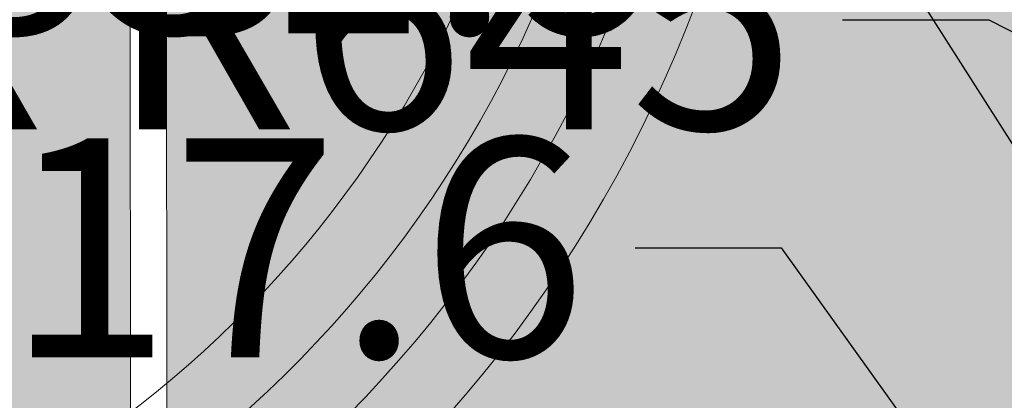
# Model space of a CAD drawing. Units: millimetres. Extents: x 11032 to 26788, y 3406 to 24505.
# Tile 26 of 78: x 18325 to 18999, y 11174 to 11434. Entities that reach past the tile are written whole.
import ezdxf

# ---------------------------------------------------------------- set-up
doc = ezdxf.new("R2010")
doc.units = ezdxf.units.MM
doc.header["$MEASUREMENT"] = 0
for name, color, linetype, lineweight in [('A-ANNO-DIMS', 2, 'Continuous', 18), ('A-ELEV-GUIT', 7, 'Continuous', 18), ('A-ELEV-GUIT-PATT', 7, 'Continuous', 13), ('A-ELEV-INLY', 8, 'Continuous', 13), ('A-ELEV-INLY-PATT', 250, 'Continuous', 13), ('A-ELEV-STRG', 7, 'Continuous', 13)]:
    doc.layers.add(name, color=color, linetype=linetype, lineweight=lineweight)
doc.styles.get("Standard").update_dxf_attribs({"font": 'arial.ttf'})
doc.dimstyles.get("Standard").update_dxf_attribs({"dimtxt": 150, "dimasz": 100, "dimexe": 10, "dimexo": 5, "dimgap": 5, "dimtad": 0, "dimtih": 1, "dimtoh": 1, "dimdec": 0, "dimzin": 0, "dimdsep": 46, "dimtxsty": 'Standard', "dimcen": 0.09, "dimadec": 0, "dimazin": 0, "dimtfac": 1, "dimtdec": 0, "dimtofl": 0, "dimtmove": 0, "dimatfit": 3, "dimfxl": 1, "dimtolj": 1, "dimtzin": 0, "dimarcsym": 0})

# ---------------------------------------------------------------- blocks, each defined once
blk = doc.blocks.new('*D36')
at = {"layer": 'A-ANNO-DIMS', "color": 0, "lineweight": -2, "transparency": 16777216}
for p, q in [((12301.26, 17115.89), (12301.26, 24416.86)), ((25397.4, 4466.4), (25397.4, 24416.86)), ((12401.26, 24406.86), (18569.2, 24406.86)), ((25297.4, 24406.86), (19129.47, 24406.86))]:
    blk.add_line(p, q, dxfattribs=at)
at = {"layer": 'A-ANNO-DIMS', "color": 0, "transparency": 16777216}
for points in [[(12401.26, 24423.52), (12401.26, 24390.19), (12301.26, 24406.86)], [(25297.4, 24423.52), (25297.4, 24390.19), (25397.4, 24406.86)]]:
    blk.add_solid(points, dxfattribs=at)
at = {"layer": 'Defpoints', "color": 0, "transparency": 16777216}
for p in [(25397.4, 24406.86), (12301.26, 17110.89), (25397.4, 4461.4)]:
    blk.add_point(p, dxfattribs=at)
at = {"layer": 'A-ANNO-DIMS', "color": 0, "transparency": 16777216, "insert": (18849.33, 24406.86), "char_height": 150, "attachment_point": 5}
blk.add_mtext('\\A1;13096', dxfattribs=at)
blk = doc.blocks.new('*D50')
at = {"layer": 'A-ANNO-DIMS', "color": 0, "lineweight": -2, "transparency": 16777216}
for p, q in [((19697.4, 16000.71), (19697.4, 3494.9)), ((17953.45, 10206.41), (17953.45, 3494.9)), ((18053.45, 3504.9), (18603.82, 3504.9)), ((19597.4, 3504.9), (19047.04, 3504.9))]:
    blk.add_line(p, q, dxfattribs=at)
at = {"layer": 'A-ANNO-DIMS', "color": 0, "transparency": 16777216}
for points in [[(18053.45, 3521.57), (18053.45, 3488.23), (17953.45, 3504.9)], [(19597.4, 3521.57), (19597.4, 3488.23), (19697.4, 3504.9)]]:
    blk.add_solid(points, dxfattribs=at)
at = {"layer": 'Defpoints', "color": 0, "transparency": 16777216}
for p in [(19697.4, 16005.71), (17953.45, 10211.41), (19697.4, 3504.9)]:
    blk.add_point(p, dxfattribs=at)
at = {"layer": 'A-ANNO-DIMS', "color": 0, "transparency": 16777216, "insert": (18825.43, 3504.9), "char_height": 150, "attachment_point": 5}
blk.add_mtext('\\A1;1744', dxfattribs=at)
blk = doc.blocks.new('*D57')
at = {"layer": 'A-ANNO-DIMS', "color": 0, "lineweight": -2, "transparency": 16777216}
for p, q in [((14994.7, 7266.4), (14994.7, 24416.86)), ((20894.7, 7266.4), (20894.7, 24416.86)), ((15094.7, 24406.86), (17715.98, 24406.86)), ((20794.7, 24406.86), (18173.42, 24406.86))]:
    blk.add_line(p, q, dxfattribs=at)
at = {"layer": 'A-ANNO-DIMS', "color": 0, "transparency": 16777216}
for points in [[(15094.7, 24423.52), (15094.7, 24390.19), (14994.7, 24406.86)], [(20794.7, 24423.52), (20794.7, 24390.19), (20894.7, 24406.86)]]:
    blk.add_solid(points, dxfattribs=at)
at = {"layer": 'Defpoints', "color": 0, "transparency": 16777216}
for p in [(20894.7, 24406.86), (14994.7, 7261.4), (20894.7, 7261.4)]:
    blk.add_point(p, dxfattribs=at)
at = {"layer": 'A-ANNO-DIMS', "color": 0, "transparency": 16777216, "insert": (17944.7, 24406.86), "char_height": 150, "attachment_point": 5}
blk.add_mtext('\\A1;5900', dxfattribs=at)
blk = doc.blocks.new('*D70')
at = {"layer": 'A-ANNO-DIMS', "color": 0, "lineweight": -2, "transparency": 16777216}
for p, q in [((18044.7, 11901.4), (17944.7, 11901.4)), ((17944.7, 11901.4), (17944.7, 10261.4)), ((17944.61, 7261.4), (17944.79, 7261.4)), ((17944.7, 7261.31), (17944.7, 7261.49))]:
    blk.add_line(p, q, dxfattribs=at)
at = {"layer": 'A-ANNO-DIMS', "color": 0, "transparency": 16777216}
blk.add_solid([(17928.04, 10261.4), (17961.37, 10261.4), (17944.7, 10161.4)], dxfattribs=at)
at = {"layer": 'Defpoints', "color": 0, "transparency": 16777216}
for p in [(17944.7, 10161.4), (17944.7, 7261.4)]:
    blk.add_point(p, dxfattribs=at)
at = {"layer": 'A-ANNO-DIMS', "color": 0, "transparency": 16777216, "insert": (18345.2, 11901.4), "char_height": 150, "attachment_point": 5}
blk.add_mtext('\\A1;R2900', dxfattribs=at)
blk = doc.blocks.new('*D78')
at = {"layer": 'A-ANNO-DIMS', "color": 0, "lineweight": -2, "transparency": 16777216}
for p, q in [((19278.06, 11833.8), (19378.06, 11833.8)), ((19378.06, 11833.8), (19386.9, 11238.32)), ((19405.52, 9979.24), (19405.7, 9979.24)), ((19405.61, 9979.15), (19405.61, 9979.33))]:
    blk.add_line(p, q, dxfattribs=at)
at = {"layer": 'A-ANNO-DIMS', "color": 0, "transparency": 16777216}
blk.add_solid([(19403.57, 11238.57), (19370.24, 11238.08), (19388.39, 11138.34)], dxfattribs=at)
at = {"layer": 'Defpoints', "color": 0, "transparency": 16777216}
for p in [(19388.39, 11138.34), (19405.61, 9979.24)]:
    blk.add_point(p, dxfattribs=at)
at = {"layer": 'A-ANNO-DIMS', "color": 0, "transparency": 16777216, "insert": (18728.26, 11833.8), "char_height": 150, "attachment_point": 5}
blk.add_mtext('\\A1;2X R1159.2', dxfattribs=at)
blk = doc.blocks.new('*D79')
at = {"layer": 'A-ANNO-DIMS', "color": 0, "lineweight": -2, "transparency": 16777216}
for p, q in [((19621.6, 11163.41), (19157.07, 10798.82)), ((19721.6, 11163.41), (19621.6, 11163.41)), ((18173, 10026.54), (18173.18, 10026.54)), ((18173.09, 10026.45), (18173.09, 10026.63))]:
    blk.add_line(p, q, dxfattribs=at)
at = {"layer": 'A-ANNO-DIMS', "color": 0, "transparency": 16777216}
blk.add_solid([(19146.78, 10811.93), (19167.36, 10785.71), (19078.4, 10737.08)], dxfattribs=at)
at = {"layer": 'Defpoints', "color": 0, "transparency": 16777216}
for p in [(19078.4, 10737.08), (18173.09, 10026.54)]:
    blk.add_point(p, dxfattribs=at)
at = {"layer": 'A-ANNO-DIMS', "color": 0, "transparency": 16777216, "insert": (20272.31, 11163.41), "char_height": 150, "attachment_point": 5}
blk.add_mtext('\\A1;2X R1150.9', dxfattribs=at)
blk = doc.blocks.new('*D80')
at = {"layer": 'A-ANNO-DIMS', "color": 0, "lineweight": -2, "transparency": 16777216}
for p, q in [((18808.09, 11500), (18908.09, 11500)), ((18908.09, 11500), (19122.53, 11163.36)), ((19623.1, 10377.38), (19623.28, 10377.38)), ((19623.19, 10377.29), (19623.19, 10377.47))]:
    blk.add_line(p, q, dxfattribs=at)
at = {"layer": 'A-ANNO-DIMS', "color": 0, "transparency": 16777216}
blk.add_solid([(19136.58, 11172.31), (19108.47, 11154.4), (19176.25, 11079.02)], dxfattribs=at)
at = {"layer": 'Defpoints', "color": 0, "transparency": 16777216}
for p in [(19176.25, 11079.02), (19623.19, 10377.38)]:
    blk.add_point(p, dxfattribs=at)
at = {"layer": 'A-ANNO-DIMS', "color": 0, "transparency": 16777216, "insert": (18315.64, 11500), "char_height": 150, "attachment_point": 5}
blk.add_mtext('\\A1;2X R831.9', dxfattribs=at)
blk = doc.blocks.new('*D81')
at = {"layer": 'A-ANNO-DIMS', "color": 0, "lineweight": -2, "transparency": 16777216}
for p, q in [((18746.01, 11278.33), (18846.01, 11278.33)), ((18846.01, 11278.33), (19073.46, 10960.86)), ((19607.77, 10214.96), (19607.95, 10214.96)), ((19607.86, 10214.87), (19607.86, 10215.05))]:
    blk.add_line(p, q, dxfattribs=at)
at = {"layer": 'A-ANNO-DIMS', "color": 0, "transparency": 16777216}
blk.add_solid([(19087.01, 10970.56), (19059.91, 10951.15), (19131.7, 10879.56)], dxfattribs=at)
at = {"layer": 'Defpoints', "color": 0, "transparency": 16777216}
for p in [(19131.7, 10879.56), (19607.86, 10214.96)]:
    blk.add_point(p, dxfattribs=at)
at = {"layer": 'A-ANNO-DIMS', "color": 0, "transparency": 16777216, "insert": (18253.76, 11278.33), "char_height": 150, "attachment_point": 5}
blk.add_mtext('\\A1;2X R817.6', dxfattribs=at)
blk = doc.blocks.new('*D83')
at = {"layer": 'A-ANNO-DIMS', "color": 0, "lineweight": -2, "transparency": 16777216}
for p, q in [((19272.33, 11150.07), (19043.23, 10964.72)), ((19372.33, 11150.07), (19272.33, 11150.07)), ((18453.97, 10488.08), (18454.15, 10488.08)), ((18454.06, 10487.99), (18454.06, 10488.17))]:
    blk.add_line(p, q, dxfattribs=at)
at = {"layer": 'A-ANNO-DIMS', "color": 0, "transparency": 16777216}
blk.add_solid([(19032.74, 10977.67), (19053.71, 10951.76), (18965.48, 10901.82)], dxfattribs=at)
at = {"layer": 'Defpoints', "color": 0, "transparency": 16777216}
for p in [(18965.48, 10901.82), (18454.06, 10488.08)]:
    blk.add_point(p, dxfattribs=at)
at = {"layer": 'A-ANNO-DIMS', "color": 0, "transparency": 16777216, "insert": (19864.78, 11150.07), "char_height": 150, "attachment_point": 5}
blk.add_mtext('\\A1;2X R657.8', dxfattribs=at)
blk = doc.blocks.new('*D84')
at = {"layer": 'A-ANNO-DIMS', "color": 0, "lineweight": -2, "transparency": 16777216}
for p, q in [((18888.04, 11434.41), (18988.04, 11434.41)), ((18988.04, 11434.41), (19243.8, 11304.14)), ((19907.6, 10966), (19907.78, 10966)), ((19907.69, 10965.91), (19907.69, 10966.09))]:
    blk.add_line(p, q, dxfattribs=at)
at = {"layer": 'A-ANNO-DIMS', "color": 0, "transparency": 16777216}
blk.add_solid([(19251.37, 11319), (19236.24, 11289.29), (19332.91, 11258.76)], dxfattribs=at)
at = {"layer": 'Defpoints', "color": 0, "transparency": 16777216}
for p in [(19332.91, 11258.76), (19907.69, 10966)]:
    blk.add_point(p, dxfattribs=at)
at = {"layer": 'A-ANNO-DIMS', "color": 0, "transparency": 16777216, "insert": (18482.56, 11434.41), "char_height": 150, "attachment_point": 5}
blk.add_mtext('\\A1;2X R645', dxfattribs=at)

msp = doc.modelspace()

# ---------------------------------------------------------------- hatches: boundary and pattern name
at = {"layer": 'A-ELEV-GUIT-PATT'}
h = msp.add_hatch(color=256, dxfattribs=at)
h.paths.add_polyline_path([(18424.39, 12337.941), (18425.299, 11185.614, 0.4683722)])
h.paths.add_polyline_path([(17502.928, 12367.48, 0.4909953), (17469.585, 11181.087)])
h.paths.add_polyline_path([(17654.236, 12452.868, 0.0477145), (17528.428, 12385.27), (17494.045, 11161.894, 0.0503453), (17622.952, 11083.922)])
h.paths.add_polyline_path([(17803.94, 12498.071, 0.0431928), (17679.468, 12462.933), (17647.696, 11072.715, 0.0458241), (17778.106, 11030.137)])
h.paths.add_polyline_path([(17950.249, 12511.239), (17829.354, 12521.528), (17803.014, 11024.905, 0.0436508), (17933.027, 11011.49)])
h.paths.add_polyline_path([(18101.906, 12494.739, 0.0426353), (17975.244, 12510.777), (17958.028, 11011.518, 0.0435176), (18087.619, 11025.142)])
h.paths.add_polyline_path([(18250.372, 12446.284, 0.0436439), (18126.849, 12488.945), (18112.671, 11030.45, 0.0462768), (18244.243, 11073.812)])
h.paths.add_polyline_path([(18399.373, 12357.869, 0.0487365), (18275.32, 12434.595), (18269.295, 11085.277, 0.0513698), (18400.312, 11165.647)])
h = msp.add_hatch(color=256, dxfattribs=at)
h.paths.add_polyline_path([(18424.244, 12523.003), (18424.291, 12463.18, -0.5273141), (18425.397, 11060.376), (18425.445, 11000.552, 0.5515566)])
h.paths.add_polyline_path([(18424.291, 12463.18), (18424.34, 12401.672, -0.4998624), (18425.349, 11121.884), (18425.397, 11060.376, 0.5273141)], flags=17)
h.paths.add_polyline_path([(18424.34, 12401.672), (18424.39, 12337.941, -0.4683722), (18425.299, 11185.614), (18425.349, 11121.884, 0.4998624)], flags=16)
at = {"layer": 'A-ELEV-INLY-PATT'}
h = msp.add_hatch(color=256, dxfattribs=at)
h.set_gradient(color2=(38, 38, 39), name='HEMISPHERICAL')
edge = h.paths.add_edge_path()
edge.add_spline(control_points=[(18425.445, 11000.552), (18458.708, 10987.38), (18550.3, 10951.111), (18655.663, 10967.984), (18775.66, 10985.753), (18767.173, 11045.69), (18820.435, 11029.121), (18856.601, 11081.429), (18910.606, 10999.748), (18944.51, 11067.805), (18993.671, 11025.073), (19010.479, 11088.113), (19112.886, 11074.83), (18997.512, 11168.165), (19020.085, 11271.149), (19186.417, 11251.458), (19043.711, 11367.761), (19195.966, 11319.856), (19164.81, 11418.359), (19240.548, 11369.352), (19291.772, 11465.595), (19340.205, 11366.103), (19400.937, 11422.431), (19448.16, 11354.501), (19470.028, 11298.294), (19504.824, 11295.807)], knot_values=[0, 0, 0, 0, 104.1926844, 286.8965309, 358.0276019, 380.9077181, 428.8178922, 462.9108054, 536.6618053, 575.7062143, 616.0072998, 661.1892288, 710.1041052, 826.2545772, 880.3446099, 992.4558514, 1059.8900815, 1142.5885686, 1188.5458396, 1228.1561193, 1314.4611862, 1376.292047, 1433.035567, 1479.0146796, 1584.2445291, 1584.2445291, 1584.2445291, 1584.2445291], degree=3, periodic=0)
edge.add_spline(control_points=[(19504.824, 11295.807), (19505.924, 11314.349), (19506.623, 11332.908), (19508.291, 11422.259), (19504.403, 11492.427), (19485.077, 11629.54), (19469.639, 11696.485), (19436.971, 11793.081), (19424.498, 11824.643), (19403.303, 11870.856), (19395.824, 11886.073), (19380.021, 11916.101), (19371.692, 11930.911), (19325.511, 12008.031), (19280.532, 12066.689), (19204.455, 12147.807), (19177.661, 12173.701), (19101.242, 12241.001), (19049.213, 12279.949), (18967.517, 12332.138), (18939.676, 12348.496), (18883.071, 12379.019), (18854.309, 12393.182), (18810.69, 12412.702), (18796.068, 12418.926), (18764.062, 12431.927), (18746.648, 12438.606), (18662.541, 12469.232), (18594.628, 12489.063), (18492.28, 12515.967), (18458.285, 12524.419), (18424.236, 12532.741)], knot_values=[45.1275191, 45.1275191, 45.1275191, 45.1275191, 98.76835, 98.76835, 303.9642424, 303.9642424, 509.1601349, 509.1601349, 611.7580811, 611.7580811, 663.0570542, 663.0570542, 714.3560273, 714.3560273, 934.0138233, 934.0138233, 1043.8427213, 1043.8427213, 1233.750961, 1233.750961, 1328.7050808, 1328.7050808, 1423.6592007, 1423.6592007, 1471.1362606, 1471.1362606, 1527.0566313, 1527.0566313, 1739.8301307, 1739.8301307, 1844.9911016, 1844.9911016, 1844.9911016, 1844.9911016], degree=3, periodic=0)
edge.add_line((18424.236, 12532.741), (18424.244, 12523.003))
edge.add_arc((17944.704, 11761.399), 900, -57.713267, 57.803626, ccw=False)
h = msp.add_hatch(color=256, dxfattribs=at)
edge = h.paths.add_edge_path()
edge.add_arc((18789.532, 11216.979), 500.762, -8.89746, 10.155345, ccw=False)
edge.add_arc((18705.433, 10826.987), 657.823, 28.173232, 28.366714, ccw=False)
edge.add_arc((19623.186, 10377.382), 831.89, 113.764176, 113.962715, ccw=False)
edge.add_arc((19859.228, 10553.861), 817.577, 119.622547, 134.325807, ccw=False)
edge.add_line((19455.113, 11264.581), (19500.813, 11245.508))
edge.add_spline(control_points=[(19500.813, 11245.508), (19502.502, 11262.23), (19503.828, 11279.011), (19504.824, 11295.807)], knot_values=[1844.9911016, 1844.9911016, 1844.9911016, 1844.9911016, 1893.583377, 1893.583377, 1893.583377, 1893.583377], degree=3, periodic=0)
edge.add_spline(control_points=[(19504.824, 11295.807), (19470.028, 11298.294), (19448.16, 11354.501), (19400.937, 11422.431), (19340.205, 11366.103), (19291.772, 11465.595), (19240.548, 11369.352), (19164.81, 11418.359), (19186.296, 11350.429), (19156.786, 11343.359), (19143.646, 11342.755)], knot_values=[1112.1151992, 1112.1151992, 1112.1151992, 1112.1151992, 1217.3450487, 1263.3241613, 1320.0676813, 1381.8985421, 1468.203609, 1507.8138887, 1553.7711596, 1584.2445291, 1584.2445291, 1584.2445291, 1584.2445291], degree=3, periodic=0)
edge.add_spline(control_points=[(19143.646, 11342.755), (19121.128, 11341.719), (19060.294, 11354.247), (19186.417, 11251.458), (19020.085, 11271.149), (18997.512, 11168.165), (19112.886, 11074.83), (19010.479, 11088.113), (18993.671, 11025.073), (18944.51, 11067.805), (18918.44, 11015.474), (18893.526, 11034.229), (18881.224, 11043.454)], knot_values=[498.2869319, 498.2869319, 498.2869319, 498.2869319, 550.5120496, 617.9462797, 730.0575212, 784.147554, 900.298026, 949.2129023, 994.3948314, 1034.6959168, 1073.7403258, 1112.1151992, 1112.1151992, 1112.1151992, 1112.1151992], degree=3, periodic=0)
edge.add_line((18881.224, 11043.454), (18869.346, 10974.891))
edge.add_line((18869.346, 10974.891), (18902.54, 10921.781))
edge.add_line((18902.54, 10921.781), (18941.204, 10941.113))
edge.add_line((18941.204, 10941.113), (18915.199, 10974.457))
edge.add_line((18915.199, 10974.457), (18926.924, 10970.549))
edge.add_line((18926.924, 10970.549), (18938.767, 10988.313))
edge.add_line((18938.767, 10988.313), (18968.047, 10954.535))
edge.add_line((18968.047, 10954.535), (18975.692, 10958.357))
edge.add_line((18975.692, 10958.357), (18976.135, 10959.096))
edge.add_line((18976.135, 10959.096), (18978.045, 10943.001))
edge.add_line((18978.045, 10943.001), (19013.524, 10902.07))
edge.add_line((19013.524, 10902.07), (19024.425, 10941.998))
edge.add_line((19024.425, 10941.998), (19024.028, 10943.168))
edge.add_line((19024.028, 10943.168), (19029.35, 10975.523))
edge.add_arc((18538.162, 10878.073), 500.762, 5.885125, 11.221492, ccw=False)
edge.add_line((19036.284, 10929.418), (19054.685, 10953.953))
edge.add_line((19054.685, 10953.953), (19042.977, 10929.937))
edge.add_line((19042.977, 10929.937), (19038.736, 10891.769))
edge.add_arc((18538.162, 10878.073), 500.762, -1.255906, 1.567263, ccw=False)
edge.add_line((19038.803, 10867.098), (19048.031, 10841.722))
edge.add_arc((19656.321, 10627.096), 645.044, 148.654173, 160.565357, ccw=False)
edge.add_line((19105.426, 10962.649), (19112.395, 11012.713))
edge.add_line((19112.395, 11012.713), (19115.073, 11014.715))
edge.add_line((19115.073, 11014.715), (19113.442, 10999.384))
edge.add_line((19113.442, 10999.384), (19142.342, 11028.004))
edge.add_line((19142.342, 11028.004), (19149.283, 10929.973))
edge.add_line((19149.283, 10929.973), (19108.422, 10916.186))
edge.add_line((19108.422, 10916.186), (19113.073, 10865.816))
edge.add_arc((19607.858, 10214.955), 817.577, 118.451894, 127.242129, ccw=False)
edge.add_line((19218.347, 10933.783), (19210.459, 10952.323))
edge.add_line((19210.459, 10952.323), (19197.255, 10940.744))
edge.add_line((19197.255, 10940.744), (19189.858, 11087.5))
edge.add_arc((19623.186, 10377.382), 831.89, 118.272924, 121.39235, ccw=False)
edge.add_line((19229.142, 11110.028), (19282.448, 11305.272))
edge = h.paths.add_edge_path()
edge.add_line((19367.737, 11024.758), (19434.4, 10983.069))
edge.add_spline(control_points=[(19434.4, 10983.069), (19439.373, 10993.952), (19444.043, 11004.999), (19449.538, 11019.041), (19450.634, 11021.898), (19451.711, 11024.763)], knot_values=[2115.1066164, 2115.1066164, 2115.1066164, 2115.1066164, 2151.0133162, 2151.0133162, 2160.1438274, 2160.1438274, 2160.1438274, 2160.1438274], degree=3, periodic=0)
edge.add_spline(control_points=[(19451.711, 11024.763), (19455.93, 11035.991), (19459.867, 11047.36), (19463.534, 11058.854)], knot_values=[2079.3353001, 2079.3353001, 2079.3353001, 2079.3353001, 2115.1066164, 2115.1066164, 2115.1066164, 2115.1066164], degree=3, periodic=0)
edge.add_spline(control_points=[(19463.534, 11058.854), (19468.26, 11073.668), (19472.539, 11088.69), (19476.401, 11103.88)], knot_values=[2033.2299396, 2033.2299396, 2033.2299396, 2033.2299396, 2079.3353001, 2079.3353001, 2079.3353001, 2079.3353001], degree=3, periodic=0)
edge.add_spline(control_points=[(19476.401, 11103.88), (19479.087, 11114.449), (19481.572, 11125.1), (19483.864, 11135.82)], knot_values=[2001.1514712, 2001.1514712, 2001.1514712, 2001.1514712, 2033.2299396, 2033.2299396, 2033.2299396, 2033.2299396], degree=3, periodic=0)
edge.add_spline(control_points=[(19483.864, 11135.82), (19485.032, 11141.283), (19486.15, 11146.764), (19487.22, 11152.261)], knot_values=[1984.803134, 1984.803134, 1984.803134, 1984.803134, 2001.1514712, 2001.1514712, 2001.1514712, 2001.1514712], degree=3, periodic=0)
edge.add_spline(control_points=[(19487.22, 11152.261), (19488.987, 11161.344), (19490.621, 11170.471), (19492.803, 11183.73), (19493.451, 11187.834), (19494.075, 11191.944)], knot_values=[1945.7202792, 1945.7202792, 1945.7202792, 1945.7202792, 1972.729714, 1972.729714, 1984.803134, 1984.803134, 1984.803134, 1984.803134], degree=3, periodic=0)
edge.add_spline(control_points=[(19494.075, 11191.944), (19496.769, 11209.693), (19499, 11227.566), (19500.813, 11245.508)], knot_values=[1893.583377, 1893.583377, 1893.583377, 1893.583377, 1945.7202792, 1945.7202792, 1945.7202792, 1945.7202792], degree=3, periodic=0)
edge.add_line((19500.813, 11245.508), (19455.113, 11264.581))
edge.add_arc((19859.228, 10553.861), 817.577, 119.622547, 134.325807)
edge.add_arc((19623.186, 10377.382), 831.89, 113.764176, 113.962715)
edge.add_arc((18705.433, 10826.987), 657.823, 28.173232, 28.366714)
edge.add_arc((18789.532, 11216.979), 500.762, 351.10254, 370.155345)
edge.add_line((19282.448, 11305.272), (19229.142, 11110.028))
edge.add_line((19229.142, 11110.028), (19195.612, 10987.217))
edge.add_line((19195.612, 10987.217), (19225.695, 10916.513))
edge.add_line((19225.695, 10916.513), (19203.742, 10925.675))
edge.add_arc((19607.858, 10214.955), 817.577, 119.622547, 127.242129)
edge.add_line((19113.073, 10865.816), (19118.592, 10806.033))
edge.add_line((19118.592, 10806.033), (19116.152, 10798.933))
edge.add_arc((19154.239, 9640.331), 1159.227, 90.197759, 91.882829, ccw=False)
edge.add_line((19150.238, 10799.552), (19134.188, 10775.477))
edge.add_line((19134.188, 10775.477), (19085.522, 10734.922))
edge.add_line((19085.522, 10734.922), (19153.4, 10705.916))
edge.add_spline(control_points=[(19153.4, 10705.916), (19170.745, 10714.126), (19187.657, 10722.977), (19204.039, 10732.444)], knot_values=[2499.4055552, 2499.4055552, 2499.4055552, 2499.4055552, 2552.2680641, 2552.2680641, 2552.2680641, 2552.2680641], degree=3, periodic=0)
edge.add_spline(control_points=[(19204.039, 10732.444), (19213.355, 10737.827), (19222.499, 10743.41), (19231.455, 10749.186)], knot_values=[2469.3445461, 2469.3445461, 2469.3445461, 2469.3445461, 2499.4055552, 2499.4055552, 2499.4055552, 2499.4055552], degree=3, periodic=0)
edge.add_spline(control_points=[(19231.455, 10749.186), (19234.005, 10750.831), (19236.54, 10752.492), (19258.2, 10766.907), (19276.431, 10780.55), (19302.142, 10802.295), (19310.441, 10809.758), (19326.448, 10825.097), (19334.153, 10832.974), (19349.373, 10849.6), (19356.856, 10858.373), (19372.633, 10878.181), (19380.78, 10889.312), (19398.77, 10915.997), (19408.257, 10931.774), (19416.985, 10947.99)], knot_values=[2199.403356, 2199.403356, 2199.403356, 2199.403356, 2207.9639593, 2207.9639593, 2273.0096212, 2273.0096212, 2305.5324521, 2305.5324521, 2338.055283, 2338.055283, 2372.4515713, 2372.4515713, 2413.8893864, 2413.8893864, 2469.3445461, 2469.3445461, 2469.3445461, 2469.3445461], degree=3, periodic=0)
edge.add_arc((18424.458, 10365.444), 1150.856, 30.410046, 34.952031)
h.paths.add_polyline_path([(18988.575, 10810.691, 0.0235998), (18922.825, 10828.133), (18914.732, 10787.669), (18923.247, 10753.608), (18960.486, 10761.559, -0.0059371), (18977.772, 10771.123)])
h.paths.add_polyline_path([(18982.222, 10880.228, 0.0284515), (18934.287, 10937.655), (18902.54, 10921.781), (18830.418, 10842.447), (18831.133, 10841.784, -0.0321768), (18922.825, 10828.133), (18926.924, 10848.629)])
h.paths.add_polyline_path([(18902.54, 10921.781), (18898.625, 10928.045), (18804.745, 10889.526), (18803.891, 10867.08), (18830.418, 10842.447)])

# ---------------------------------------------------------------- linework, layer by layer
at = {"layer": 'A-ELEV-GUIT'}
for radius, start, end in [(900, 118.96712, 57.803626), (850, 121.044036, 55.651805), (800, 123.369805, 53.162671), (750, 126.088521, 50.239355)]:
    msp.add_arc((17944.704, 11761.399), radius, start, end, dxfattribs=at)
at = {"layer": 'A-ELEV-INLY'}
for points, knots in [([(18424.232, 12537.889), (18562.977, 12503.994), (18939.42, 12405.671), (19429.901, 11996.89), (19551.657, 11366.066), (19406.266, 10676.866), (18611.174, 10531.068), (18382.465, 10854.626), (18332.323, 10949.148)], [43.9017403, 43.9017403, 43.9017403, 43.9017403, 472.2498304, 1211.2844307, 1793.6258437, 2340.5272824, 3154.1000811, 3469.5948326, 3469.5948326, 3469.5948326, 3469.5948326]), ([(18423.046, 12533.032), (18457.492, 12524.616), (18491.885, 12516.07), (18594.628, 12489.063), (18662.541, 12469.232), (18746.648, 12438.606), (18764.062, 12431.927), (18796.068, 12418.926), (18810.69, 12412.702), (18854.309, 12393.182), (18883.071, 12379.019), (18939.676, 12348.496), (18967.517, 12332.138), (19049.213, 12279.949), (19101.242, 12241.001), (19177.661, 12173.701), (19204.455, 12147.807), (19280.532, 12066.689), (19325.511, 12008.031), (19371.692, 11930.911), (19380.021, 11916.101), (19395.824, 11886.073), (19403.303, 11870.856), (19424.498, 11824.643), (19436.971, 11793.081), (19469.639, 11696.485), (19485.077, 11629.54), (19504.403, 11492.427), (19508.291, 11422.259), (19505.897, 11293.968), (19501.419, 11236.104), (19482.838, 11123.165), (19468.734, 11068.091), (19432.486, 10975.468), (19412.727, 10936.698), (19380.78, 10889.312), (19372.633, 10878.181), (19356.856, 10858.373), (19349.373, 10849.6), (19334.153, 10832.974), (19326.448, 10825.097), (19310.441, 10809.758), (19302.142, 10802.295), (19276.431, 10780.55), (19258.2, 10766.907), (19193.085, 10723.572), (19141.86, 10698.191), (19033.937, 10659.174), (18977.24, 10645.539), (18863.428, 10631.28), (18806.315, 10630.657), (18706.774, 10642.444), (18663.576, 10652.483), (18610.301, 10672.44), (18597.617, 10677.83), (18575.274, 10688.559), (18565.496, 10693.716), (18548.658, 10703.464), (18541.496, 10707.907), (18527.484, 10717.221), (18520.632, 10722.092), (18500.516, 10737.302), (18487.695, 10748.238), (18442.023, 10791.459), (18412.68, 10828.089), (18368.505, 10894.404), (18351.99, 10922.743), (18336.74, 10951.492)], [43.9017403, 43.9017403, 43.9017403, 43.9017403, 150.28849, 150.28849, 363.0619895, 363.0619895, 418.9823602, 418.9823602, 466.4594201, 466.4594201, 561.4135399, 561.4135399, 656.3676597, 656.3676597, 846.2758994, 846.2758994, 956.1047974, 956.1047974, 1175.7625934, 1175.7625934, 1227.0615665, 1227.0615665, 1278.3605397, 1278.3605397, 1380.9584859, 1380.9584859, 1586.1543783, 1586.1543783, 1791.3502707, 1791.3502707, 1957.7936992, 1957.7936992, 2124.2371277, 2124.2371277, 2254.8585156, 2254.8585156, 2296.2963307, 2296.2963307, 2330.692619, 2330.692619, 2363.21545, 2363.21545, 2395.7382809, 2395.7382809, 2460.7839427, 2460.7839427, 2617.0158229, 2617.0158229, 2773.247703, 2773.247703, 2929.4795832, 2929.4795832, 3057.0589812, 3057.0589812, 3098.1793964, 3098.1793964, 3131.5312179, 3131.5312179, 3157.1289484, 3157.1289484, 3182.7266789, 3182.7266789, 3233.9221399, 3233.9221399, 3373.2453482, 3373.2453482, 3469.5948326, 3469.5948326, 3469.5948326, 3469.5948326]), ([(18425.445, 11000.552), (18458.708, 10987.38), (18550.3, 10951.111), (18655.663, 10967.984), (18775.66, 10985.753), (18767.173, 11045.69), (18820.435, 11029.121), (18856.601, 11081.429), (18910.606, 10999.748), (18944.51, 11067.805), (18993.671, 11025.073), (19010.479, 11088.113), (19112.886, 11074.83), (18997.512, 11168.165), (19020.085, 11271.149), (19186.417, 11251.458), (19043.711, 11367.761), (19195.966, 11319.856), (19164.81, 11418.359), (19240.548, 11369.352), (19291.772, 11465.595), (19340.205, 11366.103), (19400.937, 11422.431), (19448.16, 11354.501), (19470.283, 11297.639), (19505.995, 11295.734), (19506.584, 11295.703)], [0, 0, 0, 0, 104.1926844, 286.8965309, 358.0276019, 380.9077181, 428.8178922, 462.9108054, 536.6618053, 575.7062143, 616.0072998, 661.1892288, 710.1041052, 826.2545772, 880.3446099, 992.4558514, 1059.8900815, 1142.5885686, 1188.5458396, 1228.1561193, 1314.4611862, 1376.292047, 1433.035567, 1479.0146796, 1584.2445291, 1586.0071764, 1586.0071764, 1586.0071764, 1586.0071764])]:
    msp.add_open_spline(points, degree=3, knots=knots, dxfattribs=at)
at = {"layer": 'A-ELEV-STRG'}
for p, q in [((18400.876, 10451.016), (18391.999, 21713.011)), ((18425.878, 10451.016), (18416.998, 21712.995))]:
    msp.add_line(p, q, dxfattribs=at)

# ---------------------------------------------------------------- dimensions: what is measured, and where the dimension line sits
at = {"layer": 'A-ANNO-DIMS'}
for base, p1, p2, picture, middle in [((25397.404, 24406.858), (12301.265, 17110.885), (25397.404, 4461.399), '*D36', (18849.334, 24406.858)), ((20894.704, 24406.858), (14994.704, 7261.399), (20894.704, 7261.399), '*D57', (17944.704, 24406.858)), ((19697.404, 3504.899), (17953.455, 10211.41), (19697.404, 16005.71), '*D50', (18825.429, 3504.899))]:
    dim = msp.add_linear_dim(base=base, p1=p1, p2=p2, dimstyle='Standard', override={"dimdec": 0, "dimlfac": 1, "dimrnd": 0, "dimzin": 0, "dimdsep": 46, "dimlunit": 2}, dxfattribs=at)
    dim.commit()
    dim.dimension.update_dxf_attribs({"geometry": picture, "text_midpoint": middle})
for center, mpoint, override, picture, middle in [((19405.609, 9979.237), (19388.388, 11138.336), {"dimdec": 1, "dimlfac": 1, "dimrnd": 0, "dimzin": 0, "dimdsep": 46, "dimlunit": 2}, '*D78', (18728.256, 11833.796)), ((19623.186, 10377.382), (19176.251, 11079.016), {"dimdec": 1, "dimlfac": 1, "dimrnd": 0, "dimzin": 0, "dimdsep": 46, "dimlunit": 2}, '*D80', (18315.641, 11499.997)), ((19907.691, 10966.001), (19332.909, 11258.758), {"dimdec": 0, "dimlfac": 1, "dimrnd": 0, "dimzin": 0, "dimdsep": 46, "dimlunit": 2}, '*D84', (18482.562, 11434.412)), ((19607.858, 10214.955), (19131.7, 10879.565), {"dimdec": 1, "dimlfac": 1, "dimrnd": 0, "dimzin": 0, "dimdsep": 46, "dimlunit": 2}, '*D81', (18253.761, 11278.331)), ((18173.088, 10026.538), (19078.405, 10737.081), {"dimdec": 1, "dimlfac": 1, "dimrnd": 0, "dimzin": 0, "dimdsep": 46, "dimlunit": 2}, '*D79', (20272.315, 11163.407)), ((18454.063, 10488.082), (18965.483, 10901.822), {"dimdec": 1, "dimlfac": 1, "dimrnd": 0, "dimzin": 0, "dimdsep": 46, "dimlunit": 2}, '*D83', (19864.784, 11150.066))]:
    dim = msp.add_radius_dim(center=center, mpoint=mpoint, text='2X <>', dimstyle='Standard', override=override, dxfattribs=at)
    dim.commit()
    dim.dimension.update_dxf_attribs({"geometry": picture, "text_midpoint": middle, "dimtype": 164})
dim = msp.add_radius_dim(center=(17944.704, 7261.399), mpoint=(17944.704, 10161.399), dimstyle='Standard', override={"dimdec": 0, "dimlfac": 1, "dimrnd": 0, "dimzin": 0, "dimdsep": 46, "dimlunit": 2}, dxfattribs=at)
dim.commit()
dim.dimension.update_dxf_attribs({"geometry": '*D70', "text_midpoint": (18345.202, 11901.399), "dimtype": 164})

doc.saveas('drawing.dxf')
